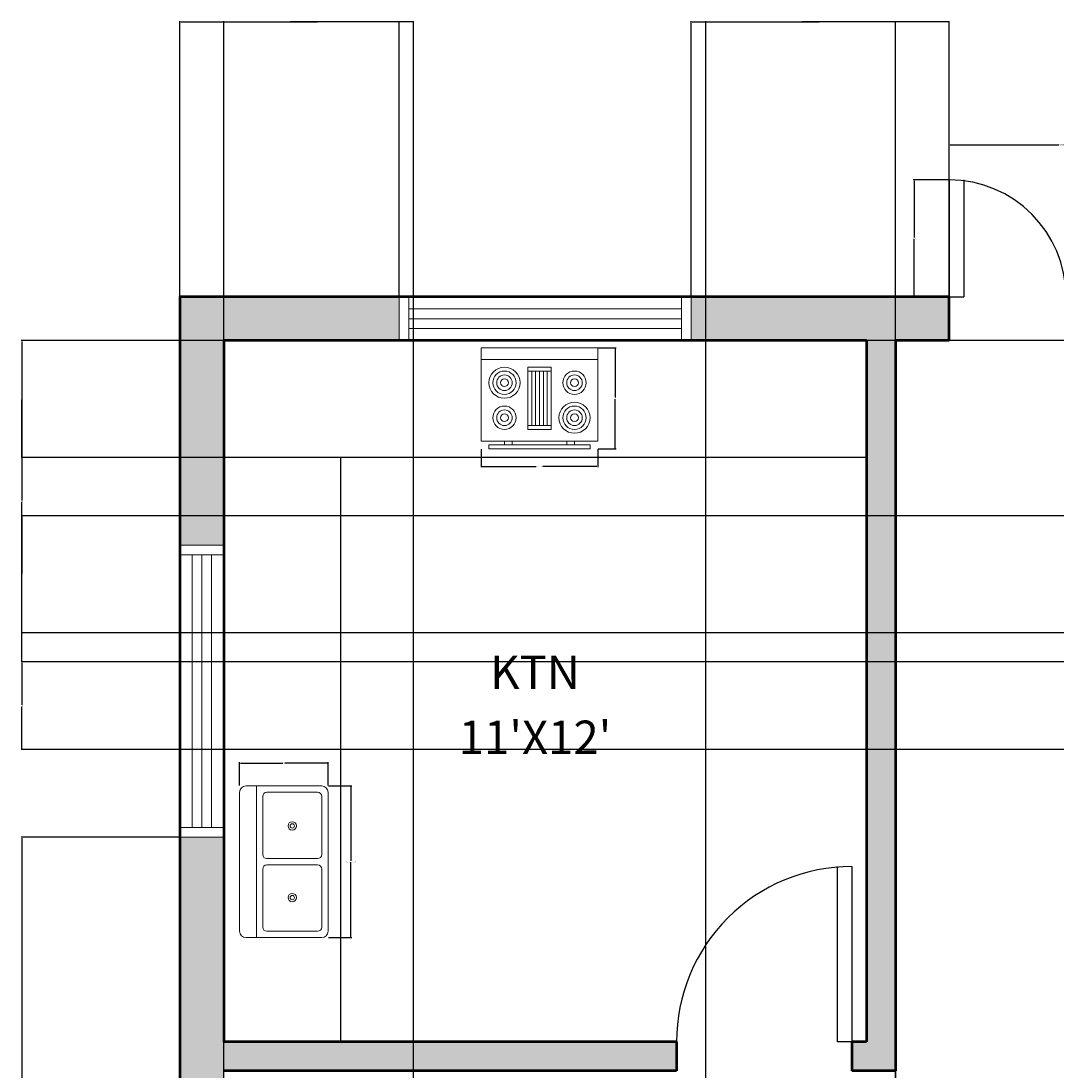
# Model space of a CAD drawing. Units: inches. Extents: x 96 to 522, y 502 to 1213.
# Tile 4 of 5: x 97 to 309, y 997 to 1213. Entities that reach past the tile are written whole.
import ezdxf

# ---------------------------------------------------------------- set-up
doc = ezdxf.new("R2010")
doc.units = ezdxf.units.IN
doc.layers.get('Defpoints').update_dxf_attribs({"color": 90})
for name, color, linetype, lineweight in [('A-ANNO-DIMS', 2, 'Continuous', 18), ('A-AREA-IDEN', 7, 'Continuous', 25), ('A-DOOR', 3, 'Continuous', 25), ('A-EQPM', 8, 'Continuous', 18), ('A-FLOR-CASE', 8, 'Continuous', 25), ('A-FLOR-FIXT', 9, 'Continuous', 18), ('A-GLAZ', 4, 'Continuous', 18), ('A-WALL', 7, 'Continuous', 50)]:
    doc.layers.add(name, color=color, linetype=linetype, lineweight=lineweight)
doc.layers.add('A-WALL-PATT', color=252, linetype='Continuous', lineweight=13, true_color=0x939598)
doc.styles.get("Standard").update_dxf_attribs({"font": 'arial.ttf'})
doc.dimstyles.get("Standard").update_dxf_attribs({"dimtxt": 0.18, "dimasz": 0.18, "dimexe": 0.18, "dimexo": 0.0625, "dimgap": 0.09, "dimtad": 0, "dimtih": 1, "dimtoh": 1, "dimdec": 4, "dimzin": 0, "dimdsep": 46, "dimtxsty": 'Standard', "dimcen": 0.09, "dimadec": 0, "dimazin": 0, "dimtfac": 1, "dimtdec": 4, "dimtofl": 0, "dimtmove": 0, "dimatfit": 3, "dimfxl": 1, "dimtolj": 1, "dimtzin": 0, "dimarcsym": 0})

# ---------------------------------------------------------------- blocks, each defined once
blk = doc.blocks.new('Range-Oven - 30 in top')
for p, q in [((0, -3), (30, -3)), ((12, -6), (18, -6)), ((13, -20), (13, -6)), ((14, -6), (14, -20)), ((15, -20), (15, -6)), ((16, -6), (16, -20)), ((17, -20), (17, -6)), ((18, -20), (12, -20)), ((6, -24), (6, -25)), ((8, -25), (8, -24)), ((22, -25), (22, -24)), ((24, -24), (24, -25))]:
    blk.add_line(p, q)
for points in [[(0, -24), (0, 0), (30, 0), (30, -24)], [(12, -21), (12, -5), (18, -5), (18, -21)], [(2, -26), (2, -25), (28, -25), (28, -26)]]:
    blk.add_lwpolyline(points, close=True)
for centre, radius in [((6, -9), 4), ((6, -9), 3), ((6, -9), 2), ((6, -9), 1), ((24, -9), 3), ((24, -9), 2), ((24, -9), 1), ((6, -18), 3), ((6, -18), 2), ((24, -18), 4), ((24, -18), 3), ((24, -18), 2), ((6, -18), 1), ((24, -18), 1)]:
    blk.add_circle(centre, radius)
blk = doc.blocks.new('Sink-double - 36 in top')
for p, q in [((-18, -4), (18, -4)), ((-0.75, -18.5), (-0.75, -6.5)), ((0.75, -6.5), (0.75, -18.5))]:
    blk.add_line(p, q)
for points in [[(-16.5, 0), (16.5, 0)], [(-18, -19.5), (-18, -1.5)], [(18, -1.5), (18, -19.5)], [(-16.5, -18.5), (-16.5, -6.5)], [(-15.5, -5.5), (-1.75, -5.5)], [(1.75, -5.5), (15.5, -5.5)], [(16.5, -6.5), (16.5, -18.5)], [(-1.75, -19.5), (-15.5, -19.5)], [(15.5, -19.5), (1.75, -19.5)], [(16.5, -21), (-16.5, -21)]]:
    blk.add_lwpolyline(points)
for centre, radius in [((-8.5, -12.5), 1), ((-8.5, -12.5), 0.5), ((8.5, -12.5), 1), ((8.5, -12.5), 0.5)]:
    blk.add_circle(centre, radius)
for centre, radius, start, end in [((-16.5, -1.5), 1.5, 90, 180), ((16.5, -1.5), 1.5, 0, 90), ((-15.5, -6.5), 1, 90, 180), ((-1.75, -6.5), 1, 0, 90), ((1.75, -6.5), 1, 90, 180), ((15.5, -6.5), 1, 0, 90), ((-16.5, -19.5), 1.5, 180, 270), ((-15.5, -18.5), 1, 180, 270), ((-1.75, -18.5), 1, 270, 0), ((1.75, -18.5), 1, 180, 270), ((15.5, -18.5), 1, 270, 0), ((16.5, -19.5), 1.5, 270, 0)]:
    blk.add_arc(centre, radius, start, end)
blk = doc.blocks.new('WIN-60IN')
for p, q in [((60, 9), (0, 9)), ((0, 9), (0, 0)), ((2, 9), (2, 0)), ((58, 0), (58, 9)), ((60, 0), (60, 9)), ((2, 6.5), (58, 6.5)), ((2, 4.5), (58, 4.5)), ((2, 2.5), (58, 2.5)), ((0, 0), (60, 0))]:
    blk.add_line(p, q)
blk = doc.blocks.new('DOOR-SGL-36IN')
for p, q in [((36, 3), (0, 3)), ((0, 0), (0, 3)), ((36, 0), (0, 0))]:
    blk.add_line(p, q)
blk.add_arc((0, 0), 36, 0, 90)
blk = doc.blocks.new('DOOR-DBL-48IN')
for p, q in [((0, 24), (0, 0)), ((3, 24), (3, 0)), ((45, 24), (45, 0)), ((48, 24), (48, 0)), ((0, 0), (3, 0)), ((48, 0), (45, 0))]:
    blk.add_line(p, q)
for centre, start, end in [((0, 0), 0, 90), ((48, 0), 90, 180)]:
    blk.add_arc(centre, 24, start, end)
blk = doc.blocks.new('*D25')
at = {"layer": 'A-ANNO-DIMS', "color": 0, "lineweight": -2, "transparency": 16777216}
for p, q in [((287.21, 1180.31), (287.21, 1187.63)), ((287.39, 1187.45), (309.72, 1187.45)), ((335.03, 1187.45), (312.7, 1187.45)), ((335.21, 1180.31), (335.21, 1187.63))]:
    blk.add_line(p, q, dxfattribs=at)
at = {"layer": 'A-ANNO-DIMS', "color": 0, "transparency": 16777216}
for points in [[(287.39, 1187.48), (287.39, 1187.42), (287.21, 1187.45)], [(335.03, 1187.48), (335.03, 1187.42), (335.21, 1187.45)]]:
    blk.add_solid(points, dxfattribs=at)
at = {"layer": 'Defpoints', "color": 0, "transparency": 16777216}
for p in [(335.21, 1187.45), (287.21, 1180.25), (335.21, 1180.25)]:
    blk.add_point(p, dxfattribs=at)
at = {"layer": 'A-ANNO-DIMS', "color": 0, "transparency": 16777216, "insert": (311.21, 1187.45), "char_height": 0.18, "attachment_point": 5}
blk.add_mtext('\\A1;DOUBLE DOOR 48 TYP.', dxfattribs=at)
blk = doc.blocks.new('*D26')
at = {"layer": 'A-ANNO-DIMS', "color": 0, "lineweight": -2, "transparency": 16777216}
for p, q in [((287.15, 1180.25), (279.83, 1180.25)), ((280.01, 1180.07), (280.01, 1168.43)), ((280.01, 1156.43), (280.01, 1168.07)), ((287.15, 1156.25), (279.83, 1156.25))]:
    blk.add_line(p, q, dxfattribs=at)
at = {"layer": 'A-ANNO-DIMS', "color": 0, "transparency": 16777216}
for points in [[(279.98, 1180.07), (280.04, 1180.07), (280.01, 1180.25)], [(279.98, 1156.43), (280.04, 1156.43), (280.01, 1156.25)]]:
    blk.add_solid(points, dxfattribs=at)
at = {"layer": 'Defpoints', "color": 0, "transparency": 16777216}
for p in [(280.01, 1180.25), (287.21, 1180.25), (287.21, 1156.25)]:
    blk.add_point(p, dxfattribs=at)
at = {"layer": 'A-ANNO-DIMS', "color": 0, "transparency": 16777216, "insert": (280.01, 1168.25), "char_height": 0.18, "attachment_point": 5}
blk.add_mtext('\\A1;24 TYP.', dxfattribs=at)
blk = doc.blocks.new('*D39')
at = {"layer": 'A-ANNO-DIMS', "color": 0, "lineweight": -2, "transparency": 16777216}
for p, q in [((191.07, 1124.95), (191.07, 1121.24)), ((215.05, 1124.95), (215.05, 1121.24)), ((191.25, 1121.42), (202.36, 1121.42)), ((214.87, 1121.42), (203.76, 1121.42))]:
    blk.add_line(p, q, dxfattribs=at)
at = {"layer": 'A-ANNO-DIMS', "color": 0, "transparency": 16777216}
for points in [[(191.25, 1121.45), (191.25, 1121.39), (191.07, 1121.42)], [(214.87, 1121.45), (214.87, 1121.39), (215.05, 1121.42)]]:
    blk.add_solid(points, dxfattribs=at)
at = {"layer": 'Defpoints', "color": 0, "transparency": 16777216}
for p in [(191.07, 1125.01), (215.05, 1125.01), (215.05, 1121.42)]:
    blk.add_point(p, dxfattribs=at)
at = {"layer": 'A-ANNO-DIMS', "color": 0, "transparency": 16777216, "insert": (203.06, 1121.42), "char_height": 0.18, "attachment_point": 5}
blk.add_mtext('\\A1;RANGE 24', dxfattribs=at)
blk = doc.blocks.new('*D40')
at = {"layer": 'A-ANNO-DIMS', "color": 0, "lineweight": -2, "transparency": 16777216}
for p, q in [((215.11, 1145.79), (218.82, 1145.79)), ((218.64, 1145.61), (218.64, 1135.58)), ((218.64, 1125.19), (218.64, 1135.22)), ((215.11, 1125.01), (218.82, 1125.01))]:
    blk.add_line(p, q, dxfattribs=at)
at = {"layer": 'A-ANNO-DIMS', "color": 0, "transparency": 16777216}
for points in [[(218.61, 1145.61), (218.67, 1145.61), (218.64, 1145.79)], [(218.61, 1125.19), (218.67, 1125.19), (218.64, 1125.01)]]:
    blk.add_solid(points, dxfattribs=at)
at = {"layer": 'Defpoints', "color": 0, "transparency": 16777216}
for p in [(215.05, 1145.79), (218.64, 1145.79), (215.05, 1125.01)]:
    blk.add_point(p, dxfattribs=at)
at = {"layer": 'A-ANNO-DIMS', "color": 0, "transparency": 16777216, "insert": (218.64, 1135.4), "char_height": 0.18, "attachment_point": 5}
blk.add_mtext('\\A1;21', dxfattribs=at)
blk = doc.blocks.new('*D41')
at = {"layer": 'A-ANNO-DIMS', "color": 0, "lineweight": -2, "transparency": 16777216}
for p, q in [((159.7, 1055.81), (164.49, 1055.81)), ((164.31, 1055.63), (164.31, 1040.41)), ((164.31, 1024.82), (164.31, 1040.04)), ((159.7, 1024.64), (164.49, 1024.64))]:
    blk.add_line(p, q, dxfattribs=at)
at = {"layer": 'A-ANNO-DIMS', "color": 0, "transparency": 16777216}
for points in [[(164.28, 1055.63), (164.34, 1055.63), (164.31, 1055.81)], [(164.28, 1024.82), (164.34, 1024.82), (164.31, 1024.64)]]:
    blk.add_solid(points, dxfattribs=at)
at = {"layer": 'Defpoints', "color": 0, "transparency": 16777216}
for p in [(159.64, 1055.81), (164.31, 1055.81), (159.64, 1024.64)]:
    blk.add_point(p, dxfattribs=at)
at = {"layer": 'A-ANNO-DIMS', "color": 0, "transparency": 16777216, "insert": (164.31, 1040.22), "char_height": 0.18, "attachment_point": 5}
blk.add_mtext('\\A1;DOUBLE SINK 31', dxfattribs=at)
blk = doc.blocks.new('*D42')
at = {"layer": 'A-ANNO-DIMS', "color": 0, "lineweight": -2, "transparency": 16777216}
for p, q in [((141.45, 1055.87), (141.45, 1060.67)), ((141.63, 1060.49), (150.34, 1060.49)), ((159.46, 1060.49), (150.76, 1060.49)), ((159.64, 1055.87), (159.64, 1060.67))]:
    blk.add_line(p, q, dxfattribs=at)
at = {"layer": 'A-ANNO-DIMS', "color": 0, "transparency": 16777216}
for points in [[(141.63, 1060.52), (141.63, 1060.46), (141.45, 1060.49)], [(159.46, 1060.52), (159.46, 1060.46), (159.64, 1060.49)]]:
    blk.add_solid(points, dxfattribs=at)
at = {"layer": 'Defpoints', "color": 0, "transparency": 16777216}
for p in [(141.45, 1060.49), (141.45, 1055.81), (159.64, 1055.81)]:
    blk.add_point(p, dxfattribs=at)
at = {"layer": 'A-ANNO-DIMS', "color": 0, "transparency": 16777216, "insert": (150.55, 1060.49), "char_height": 0.18, "attachment_point": 5}
blk.add_mtext('\\A1;18', dxfattribs=at)
blk = doc.blocks.new('*D50')
at = {"layer": 'A-ANNO-DIMS', "color": 0, "lineweight": -2, "transparency": 16777216}
for p, q in [((129.21, 1156.31), (129.21, 1212.88)), ((129.39, 1212.7), (151.49, 1212.7)), ((174.03, 1212.7), (151.93, 1212.7)), ((174.21, 1156.31), (174.21, 1212.88))]:
    blk.add_line(p, q, dxfattribs=at)
at = {"layer": 'A-ANNO-DIMS', "color": 0, "transparency": 16777216}
for points in [[(129.39, 1212.73), (129.39, 1212.67), (129.21, 1212.7)], [(174.03, 1212.73), (174.03, 1212.67), (174.21, 1212.7)]]:
    blk.add_solid(points, dxfattribs=at)
at = {"layer": 'Defpoints', "color": 0, "transparency": 16777216}
for p in [(174.21, 1212.7), (129.21, 1156.25), (174.21, 1156.25)]:
    blk.add_point(p, dxfattribs=at)
at = {"layer": 'A-ANNO-DIMS', "color": 0, "transparency": 16777216, "insert": (151.71, 1212.7), "char_height": 0.18, "attachment_point": 5}
blk.add_mtext('\\A1;45', dxfattribs=at)
blk = doc.blocks.new('*D51')
at = {"layer": 'A-ANNO-DIMS', "color": 0, "lineweight": -2, "transparency": 16777216}
for p, q in [((234.21, 1156.31), (234.21, 1212.88)), ((234.39, 1212.7), (260.49, 1212.7)), ((287.03, 1212.7), (260.93, 1212.7)), ((287.21, 1156.31), (287.21, 1212.88))]:
    blk.add_line(p, q, dxfattribs=at)
at = {"layer": 'A-ANNO-DIMS', "color": 0, "transparency": 16777216}
for points in [[(234.39, 1212.73), (234.39, 1212.67), (234.21, 1212.7)], [(287.03, 1212.73), (287.03, 1212.67), (287.21, 1212.7)]]:
    blk.add_solid(points, dxfattribs=at)
at = {"layer": 'Defpoints', "color": 0, "transparency": 16777216}
for p in [(287.21, 1212.7), (234.21, 1156.25), (287.21, 1156.25)]:
    blk.add_point(p, dxfattribs=at)
at = {"layer": 'A-ANNO-DIMS', "color": 0, "transparency": 16777216, "insert": (260.71, 1212.7), "char_height": 0.18, "attachment_point": 5}
blk.add_mtext('\\A1;53', dxfattribs=at)
blk = doc.blocks.new('*D53')
at = {"layer": 'A-ANNO-DIMS', "color": 0, "lineweight": -2, "transparency": 16777216}
for p, q in [((138.21, 661.31), (138.21, 1212.88)), ((138.39, 1212.7), (157.49, 1212.7)), ((177.03, 1212.7), (157.93, 1212.7)), ((177.21, 661.31), (177.21, 1212.88))]:
    blk.add_line(p, q, dxfattribs=at)
at = {"layer": 'A-ANNO-DIMS', "color": 0, "transparency": 16777216}
for points in [[(138.39, 1212.73), (138.39, 1212.67), (138.21, 1212.7)], [(177.03, 1212.73), (177.03, 1212.67), (177.21, 1212.7)]]:
    blk.add_solid(points, dxfattribs=at)
at = {"layer": 'Defpoints', "color": 0, "transparency": 16777216}
for p in [(177.21, 1212.7), (138.21, 661.25), (177.21, 661.25)]:
    blk.add_point(p, dxfattribs=at)
at = {"layer": 'A-ANNO-DIMS', "color": 0, "transparency": 16777216, "insert": (157.71, 1212.7), "char_height": 0.18, "attachment_point": 5}
blk.add_mtext('\\A1;39', dxfattribs=at)
blk = doc.blocks.new('*D54')
at = {"layer": 'A-ANNO-DIMS', "color": 0, "lineweight": -2, "transparency": 16777216}
for p, q in [((237.21, 661.31), (237.21, 1212.88)), ((237.39, 1212.7), (256.49, 1212.7)), ((276.03, 1212.7), (256.93, 1212.7)), ((276.21, 661.31), (276.21, 1212.88))]:
    blk.add_line(p, q, dxfattribs=at)
at = {"layer": 'A-ANNO-DIMS', "color": 0, "transparency": 16777216}
for points in [[(237.39, 1212.73), (237.39, 1212.67), (237.21, 1212.7)], [(276.03, 1212.73), (276.03, 1212.67), (276.21, 1212.7)]]:
    blk.add_solid(points, dxfattribs=at)
at = {"layer": 'Defpoints', "color": 0, "transparency": 16777216}
for p in [(276.21, 1212.7), (237.21, 661.25), (276.21, 661.25)]:
    blk.add_point(p, dxfattribs=at)
at = {"layer": 'A-ANNO-DIMS', "color": 0, "transparency": 16777216, "insert": (256.71, 1212.7), "char_height": 0.18, "attachment_point": 5}
blk.add_mtext('\\A1;39', dxfattribs=at)
blk = doc.blocks.new('*D59')
at = {"layer": 'A-ANNO-DIMS', "color": 0, "lineweight": -2, "transparency": 16777216}
for p, q in [((129.15, 1045.25), (96.58, 1045.25)), ((96.76, 1045.07), (96.76, 982.43)), ((96.76, 919.43), (96.76, 982.07)), ((129.15, 919.25), (96.58, 919.25))]:
    blk.add_line(p, q, dxfattribs=at)
at = {"layer": 'A-ANNO-DIMS', "color": 0, "transparency": 16777216}
for points in [[(96.73, 1045.07), (96.79, 1045.07), (96.76, 1045.25)], [(96.73, 919.43), (96.79, 919.43), (96.76, 919.25)]]:
    blk.add_solid(points, dxfattribs=at)
at = {"layer": 'Defpoints', "color": 0, "transparency": 16777216}
for p in [(96.76, 1045.25), (129.21, 1045.25), (129.21, 919.25)]:
    blk.add_point(p, dxfattribs=at)
at = {"layer": 'A-ANNO-DIMS', "color": 0, "transparency": 16777216, "insert": (96.76, 982.25), "char_height": 0.18, "attachment_point": 5}
blk.add_mtext('\\A1;126', dxfattribs=at)
blk = doc.blocks.new('*D63')
at = {"layer": 'A-ANNO-DIMS', "color": 0, "lineweight": -2, "transparency": 16777216}
for p, q in [((480.15, 1081.25), (96.58, 1081.25)), ((96.76, 1081.07), (96.76, 1072.43)), ((96.76, 1063.43), (96.76, 1072.07)), ((480.15, 1063.25), (96.58, 1063.25))]:
    blk.add_line(p, q, dxfattribs=at)
at = {"layer": 'A-ANNO-DIMS', "color": 0, "transparency": 16777216}
for points in [[(96.73, 1081.07), (96.79, 1081.07), (96.76, 1081.25)], [(96.73, 1063.43), (96.79, 1063.43), (96.76, 1063.25)]]:
    blk.add_solid(points, dxfattribs=at)
at = {"layer": 'Defpoints', "color": 0, "transparency": 16777216}
for p in [(96.76, 1081.25), (480.21, 1081.25), (480.21, 1063.25)]:
    blk.add_point(p, dxfattribs=at)
at = {"layer": 'A-ANNO-DIMS', "color": 0, "transparency": 16777216, "insert": (96.76, 1072.25), "char_height": 0.18, "attachment_point": 5}
blk.add_mtext('\\A1;18', dxfattribs=at)
blk = doc.blocks.new('*D64')
at = {"layer": 'A-ANNO-DIMS', "color": 0, "lineweight": -2, "transparency": 16777216}
for p, q in [((480.15, 1111.25), (96.58, 1111.25)), ((96.76, 1111.07), (96.76, 1099.43)), ((96.76, 1087.43), (96.76, 1099.07)), ((480.15, 1087.25), (96.58, 1087.25))]:
    blk.add_line(p, q, dxfattribs=at)
at = {"layer": 'A-ANNO-DIMS', "color": 0, "transparency": 16777216}
for points in [[(96.73, 1111.07), (96.79, 1111.07), (96.76, 1111.25)], [(96.73, 1087.43), (96.79, 1087.43), (96.76, 1087.25)]]:
    blk.add_solid(points, dxfattribs=at)
at = {"layer": 'Defpoints', "color": 0, "transparency": 16777216}
for p in [(96.76, 1111.25), (480.21, 1111.25), (480.21, 1087.25)]:
    blk.add_point(p, dxfattribs=at)
at = {"layer": 'A-ANNO-DIMS', "color": 0, "transparency": 16777216, "insert": (96.76, 1099.25), "char_height": 0.18, "attachment_point": 5}
blk.add_mtext('\\A1;24', dxfattribs=at)
blk = doc.blocks.new('*D66')
at = {"layer": 'A-ANNO-DIMS', "color": 0, "lineweight": -2, "transparency": 16777216}
for p, q in [((330.21, 1033.19), (330.21, 501.62)), ((276.21, 997.19), (276.21, 501.62)), ((276.39, 501.8), (302.99, 501.8)), ((330.03, 501.8), (303.43, 501.8))]:
    blk.add_line(p, q, dxfattribs=at)
at = {"layer": 'A-ANNO-DIMS', "color": 0, "transparency": 16777216}
for points in [[(276.39, 501.83), (276.39, 501.77), (276.21, 501.8)], [(330.03, 501.83), (330.03, 501.77), (330.21, 501.8)]]:
    blk.add_solid(points, dxfattribs=at)
at = {"layer": 'Defpoints', "color": 0, "transparency": 16777216}
for p in [(330.21, 1033.25), (276.21, 997.25), (330.21, 501.8)]:
    blk.add_point(p, dxfattribs=at)
at = {"layer": 'A-ANNO-DIMS', "color": 0, "transparency": 16777216, "insert": (303.21, 501.8), "char_height": 0.18, "attachment_point": 5}
blk.add_mtext('\\A1;54', dxfattribs=at)
blk = doc.blocks.new('*D69')
at = {"layer": 'A-ANNO-DIMS', "color": 0, "lineweight": -2, "transparency": 16777216}
for p, q in [((138.15, 1147.25), (96.58, 1147.25)), ((96.76, 1147.07), (96.76, 1135.43)), ((96.76, 1123.43), (96.76, 1135.07)), ((162.15, 1123.25), (96.58, 1123.25))]:
    blk.add_line(p, q, dxfattribs=at)
at = {"layer": 'A-ANNO-DIMS', "color": 0, "transparency": 16777216}
for points in [[(96.73, 1147.07), (96.79, 1147.07), (96.76, 1147.25)], [(96.73, 1123.43), (96.79, 1123.43), (96.76, 1123.25)]]:
    blk.add_solid(points, dxfattribs=at)
at = {"layer": 'Defpoints', "color": 0, "transparency": 16777216}
for p in [(138.21, 1147.25), (96.76, 1123.25), (162.21, 1123.25)]:
    blk.add_point(p, dxfattribs=at)
at = {"layer": 'A-ANNO-DIMS', "color": 0, "transparency": 16777216, "insert": (96.76, 1135.25), "char_height": 0.18, "attachment_point": 5}
blk.add_mtext('\\A1;24', dxfattribs=at)
blk = doc.blocks.new('*D71')
at = {"layer": 'A-ANNO-DIMS', "color": 0, "lineweight": -2, "transparency": 16777216}
for p, q in [((338.15, 1147.25), (96.58, 1147.25)), ((96.76, 1147.07), (96.76, 1114.43)), ((96.76, 1081.43), (96.76, 1114.07)), ((338.15, 1081.25), (96.58, 1081.25))]:
    blk.add_line(p, q, dxfattribs=at)
at = {"layer": 'A-ANNO-DIMS', "color": 0, "transparency": 16777216}
for points in [[(96.73, 1147.07), (96.79, 1147.07), (96.76, 1147.25)], [(96.73, 1081.43), (96.79, 1081.43), (96.76, 1081.25)]]:
    blk.add_solid(points, dxfattribs=at)
at = {"layer": 'Defpoints', "color": 0, "transparency": 16777216}
for p in [(96.76, 1147.25), (338.21, 1147.25), (338.21, 1081.25)]:
    blk.add_point(p, dxfattribs=at)
at = {"layer": 'A-ANNO-DIMS', "color": 0, "transparency": 16777216, "insert": (96.76, 1114.25), "char_height": 0.18, "attachment_point": 5}
blk.add_mtext('\\A1;66', dxfattribs=at)

msp = doc.modelspace()

# ---------------------------------------------------------------- hatches: boundary and pattern name
at = {"layer": 'A-WALL-PATT'}
h = msp.add_hatch(color=256, dxfattribs=at)
h.dxf.hatch_style = 1
h.paths.add_polyline_path([(174.2111, 1156.2511), (129.2111, 1156.2511), (129.2111, 1105.2511), (138.2111, 1105.2511), (138.2111, 1147.2511), (174.2111, 1147.2511)])
h.paths.add_polyline_path([(287.2111, 1156.2511), (234.2111, 1156.2511), (234.2111, 1147.2511), (270.2111, 1147.2511), (270.2111, 1003.2511), (267.2111, 1003.2511), (267.2111, 997.2511), (276.2111, 997.2511), (276.2111, 1147.2511), (287.2111, 1147.2511)])
h.paths.add_polyline_path([(342.2111, 1156.2511), (335.2111, 1156.2511), (335.2111, 1147.2511), (338.2111, 1147.2511), (338.2111, 1081.2511), (342.2111, 1081.2511), (342.2111, 1147.2511)])
h.paths.add_polyline_path([(489.2111, 1156.2511), (402.2111, 1156.2511), (402.2111, 1147.2511), (402.2111, 1141.2511), (408.2111, 1141.2511), (408.2111, 1147.2511), (480.2111, 1147.2511), (480.2111, 1123.2511), (489.2111, 1123.2511)])
h.paths.add_polyline_path([(489.2111, 1111.2511), (480.2111, 1111.2511), (480.2111, 1087.2511), (408.2111, 1087.2511), (408.2111, 1111.2511), (402.2111, 1111.2511), (402.2111, 1066.2511), (408.2111, 1066.2511), (408.2111, 1081.2511), (480.2111, 1081.2511), (480.2111, 1063.2511), (489.2111, 1063.2511)])
h.paths.add_polyline_path([(489.2111, 1051.2511), (480.2111, 1051.2511), (480.2111, 1033.2511), (408.2111, 1033.2511), (408.2111, 1036.2511), (402.2111, 1036.2511), (402.2111, 1033.2511), (338.2111, 1033.2511), (330.2111, 1033.2511), (330.2111, 923.2511), (336.2111, 923.2511), (336.2111, 1027.2511), (338.2111, 1027.2511), (402.2111, 1027.2511), (480.2111, 1027.2511), (480.2111, 973.2511), (489.2111, 973.2511)])
h.paths.add_polyline_path([(489.2111, 913.2511), (480.2111, 913.2511), (480.2111, 859.2511), (429.2111, 859.2511), (429.2111, 853.2511), (480.2111, 853.2511), (480.2111, 829.2511), (489.2111, 829.2511)])
h.paths.add_polyline_path([(489.2111, 817.2511), (480.2111, 817.2511), (480.2111, 793.2511), (402.2111, 793.2511), (396.2111, 793.2511), (396.2111, 853.2511), (399.2111, 853.2511), (399.2111, 859.2511), (338.2111, 859.2511), (336.2111, 859.2511), (336.2111, 877.2511), (336.2111, 883.2511), (336.2111, 887.2511), (330.2111, 887.2511), (330.2111, 883.2511), (326.2111, 883.2511), (326.2111, 877.2511), (330.2111, 877.2511), (330.2111, 853.2511), (338.2111, 853.2511), (390.2111, 853.2511), (390.2111, 793.2511), (387.2111, 793.2511), (387.2111, 787.2511), (402.2111, 787.2511), (480.2111, 787.2511), (480.2111, 754.2511), (489.2111, 754.2511)])
h.paths.add_polyline_path([(489.2111, 694.2511), (480.2111, 694.2511), (480.2111, 661.2511), (432.2111, 661.2511), (432.2111, 652.2511), (480.2111, 652.2511), (480.2111, 543.2511), (333.2111, 543.2511), (333.2111, 534.2511), (489.2111, 534.2511), (489.2111, 652.2511)])
h.paths.add_polyline_path([(372.2111, 661.2511), (336.2111, 661.2511), (336.2111, 787.2511), (338.2111, 787.2511), (351.2111, 787.2511), (351.2111, 793.2511), (338.2111, 793.2511), (330.2111, 793.2511), (330.2111, 661.2511), (324.2111, 661.2511), (324.2111, 652.2511), (372.2111, 652.2511)])
h.paths.add_polyline_path([(138.2111, 680.6946), (129.2111, 680.6946), (129.2111, 652.2511), (177.2111, 652.2511), (177.2111, 661.2511), (138.2111, 661.2511)])
h.paths.add_polyline_path([(276.2111, 661.2511), (237.2111, 661.2511), (237.2111, 652.2511), (276.2111, 652.2511)])
h.paths.add_polyline_path([(138.2111, 803.1393), (129.2111, 803.1393), (129.2111, 740.6946), (138.2111, 740.6946)])
h.paths.add_polyline_path([(138.2111, 907.2511), (129.2111, 907.2511), (129.2111, 863.1393), (138.2111, 863.1393), (138.2111, 877.2511), (276.2111, 877.2511), (276.2111, 883.2511), (204.2111, 883.2511), (204.2111, 886.2511), (198.2111, 886.2511), (198.2111, 883.2511), (138.2111, 883.2511)])
h.paths.add_polyline_path([(138.2111, 943.2511), (198.2111, 943.2511), (198.2111, 916.2511), (204.2111, 916.2511), (204.2111, 949.2511), (138.2111, 949.2511), (138.2111, 997.2511), (231.2111, 997.2511), (231.2111, 1003.2511), (138.2111, 1003.2511), (138.2111, 1045.2511), (129.2111, 1045.2511), (129.2111, 919.2511), (138.2111, 919.2511)])

# ---------------------------------------------------------------- linework, layer by layer
at = {"layer": 'A-FLOR-CASE'}
for p, q in [((162.2111, 1123.2511), (162.2111, 1003.2511)), ((270.2111, 1123.2511), (162.2111, 1123.2511))]:
    msp.add_line(p, q, dxfattribs=at)
at = {"layer": 'A-WALL'}
for p, q in [((287.2111, 1147.2511), (287.2111, 1156.2511)), ((138.2111, 1147.2511), (138.2111, 1003.2511)), ((270.2111, 1147.2511), (138.2111, 1147.2511)), ((270.2111, 1147.2511), (270.2111, 1003.2511)), ((276.2111, 1147.2511), (276.2111, 997.2511)), ((287.2111, 1147.2511), (276.2111, 1147.2511)), ((231.2111, 1003.2511), (138.2111, 1003.2511)), ((231.2111, 1003.2511), (231.2111, 997.2511)), ((270.2111, 1003.2511), (267.2111, 1003.2511)), ((267.2111, 1003.2511), (267.2111, 997.2511)), ((231.2111, 997.2511), (138.2111, 997.2511)), ((276.2111, 997.2511), (267.2111, 997.2511))]:
    msp.add_line(p, q, dxfattribs=at)
msp.add_lwpolyline([(287.2111, 1156.2511), (129.2111, 1156.2511), (129.2111, 652.2511), (276.2111, 652.2511)], dxfattribs=at)

# ---------------------------------------------------------------- block references
at = {"layer": 'A-DOOR'}
msp.add_blockref('DOOR-DBL-48IN', (287.2111, 1156.2511), dxfattribs=at)
at = {"layer": 'A-DOOR', "rotation": 89.99999999999935}
msp.add_blockref('DOOR-SGL-36IN', (267.2111, 1003.2511), dxfattribs=at)
at = {"layer": 'A-EQPM', "xscale": 0.7992276984863426, "yscale": 0.7992276984863426, "zscale": 0.7992276984863426}
msp.add_blockref('Range-Oven - 30 in top', (191.071, 1145.7918), dxfattribs=at)
at = {"layer": 'A-FLOR-FIXT', "xscale": 0.865945991670747, "yscale": 0.865945991670747, "zscale": 0.865945991670747, "rotation": 90}
msp.add_blockref('Sink-double - 36 in top', (141.4539, 1040.2243), dxfattribs=at)
at = {"layer": 'A-GLAZ'}
for p, rotation in [((234.2111, 1156.2511), 180), ((138.2111, 1045.2511), 89.99999999999982)]:
    msp.add_blockref('WIN-60IN', p, dxfattribs=dict(at, rotation=rotation))

# ---------------------------------------------------------------- texts
at = {"layer": 'A-AREA-IDEN', "char_height": 6.85818, "attachment_point": 1}
for s, insert in [('KTN', (192.9321, 1082.5761)), ("11'X12'", (186.4882, 1069.2118))]:
    msp.add_mtext_dynamic_manual_height_columns(s, width=37.606817, gutter_width=34.2909, heights=[0], dxfattribs=dict(at, insert=insert))

# ---------------------------------------------------------------- dimensions: what is measured, and where the dimension line sits
at = {"layer": 'A-ANNO-DIMS'}
for base, p1, p2, picture, middle in [((174.2111, 1212.7011), (129.2111, 1156.2511), (174.2111, 1156.2511), '*D50', (151.7111, 1212.7011)), ((177.2111, 1212.7011), (138.2111, 661.2511), (177.2111, 661.2511), '*D53', (157.7111, 1212.7011)), ((287.2111, 1212.7011), (234.2111, 1156.2511), (287.2111, 1156.2511), '*D51', (260.7111, 1212.7011)), ((276.2111, 1212.7011), (237.2111, 661.2511), (276.2111, 661.2511), '*D54', (256.7111, 1212.7011)), ((330.2111, 501.8011), (276.2111, 997.2511), (330.2111, 1033.2511), '*D66', (303.2111, 501.8011))]:
    dim = msp.add_linear_dim(base=base, p1=p1, p2=p2, dimstyle='Standard', override={"dimdec": 0, "dimlfac": 1, "dimrnd": 0, "dimzin": 0, "dimdsep": 46, "dimlunit": 2}, dxfattribs=at)
    dim.commit()
    dim.dimension.update_dxf_attribs({"geometry": picture, "text_midpoint": middle})
for base, p1, p2, text, picture, middle in [((335.2111, 1187.4511), (287.2111, 1180.2511), (335.2111, 1180.2511), 'DOUBLE DOOR <> TYP.', '*D25', (311.2111, 1187.4511)), ((215.0478, 1121.4153), (191.071, 1125.0119), (215.0478, 1125.0119), 'RANGE <>', '*D39', (203.0594, 1121.4153))]:
    dim = msp.add_linear_dim(base=base, p1=p1, p2=p2, text=text, dimstyle='Standard', override={"dimdec": 0, "dimlfac": 1, "dimrnd": 0, "dimzin": 0, "dimdsep": 46, "dimlunit": 2}, dxfattribs=at)
    dim.commit()
    dim.dimension.update_dxf_attribs({"geometry": picture, "text_midpoint": middle})
for base, p1, p2, text, picture, middle in [((280.0111, 1180.2511), (287.2111, 1156.2511), (287.2111, 1180.2511), '<> TYP.', '*D26', (280.0111, 1168.2511)), ((164.3149, 1055.8113), (159.6388, 1024.6372), (159.6388, 1055.8113), 'DOUBLE SINK <>', '*D41', (164.3149, 1040.2243))]:
    dim = msp.add_linear_dim(base=base, p1=p1, p2=p2, angle=90, text=text, dimstyle='Standard', override={"dimdec": 0, "dimlfac": 1, "dimrnd": 0, "dimzin": 0, "dimdsep": 46, "dimlunit": 2}, dxfattribs=at)
    dim.commit()
    dim.dimension.update_dxf_attribs({"geometry": picture, "text_midpoint": middle})
for base, p1, p2, angle, picture, middle in [((96.7611, 1123.2511), (138.2111, 1147.2511), (162.2111, 1123.2511), 90, '*D69', (96.7611, 1135.2511)), ((96.7611, 1147.2511), (338.2111, 1081.2511), (338.2111, 1147.2511), 90, '*D71', (96.7611, 1114.2511)), ((218.6443, 1145.7918), (215.0478, 1125.0119), (215.0478, 1145.7918), 90, '*D40', (218.6443, 1135.4018)), ((96.7611, 1111.2511), (480.2111, 1087.2511), (480.2111, 1111.2511), 90, '*D64', (96.7611, 1099.2511)), ((96.7611, 1081.2511), (480.2111, 1063.2511), (480.2111, 1081.2511), 90, '*D63', (96.7611, 1072.2511)), ((141.4539, 1060.4874), (159.6388, 1055.8113), (141.4539, 1055.8113), 180, '*D42', (150.5464, 1060.4874)), ((96.7611, 1045.2511), (129.2111, 919.2511), (129.2111, 1045.2511), 90, '*D59', (96.7611, 982.2511))]:
    dim = msp.add_linear_dim(base=base, p1=p1, p2=p2, angle=angle, dimstyle='Standard', override={"dimdec": 0, "dimlfac": 1, "dimrnd": 0, "dimzin": 0, "dimdsep": 46, "dimlunit": 2}, dxfattribs=at)
    dim.commit()
    dim.dimension.update_dxf_attribs({"geometry": picture, "text_midpoint": middle})

doc.saveas('drawing.dxf')
